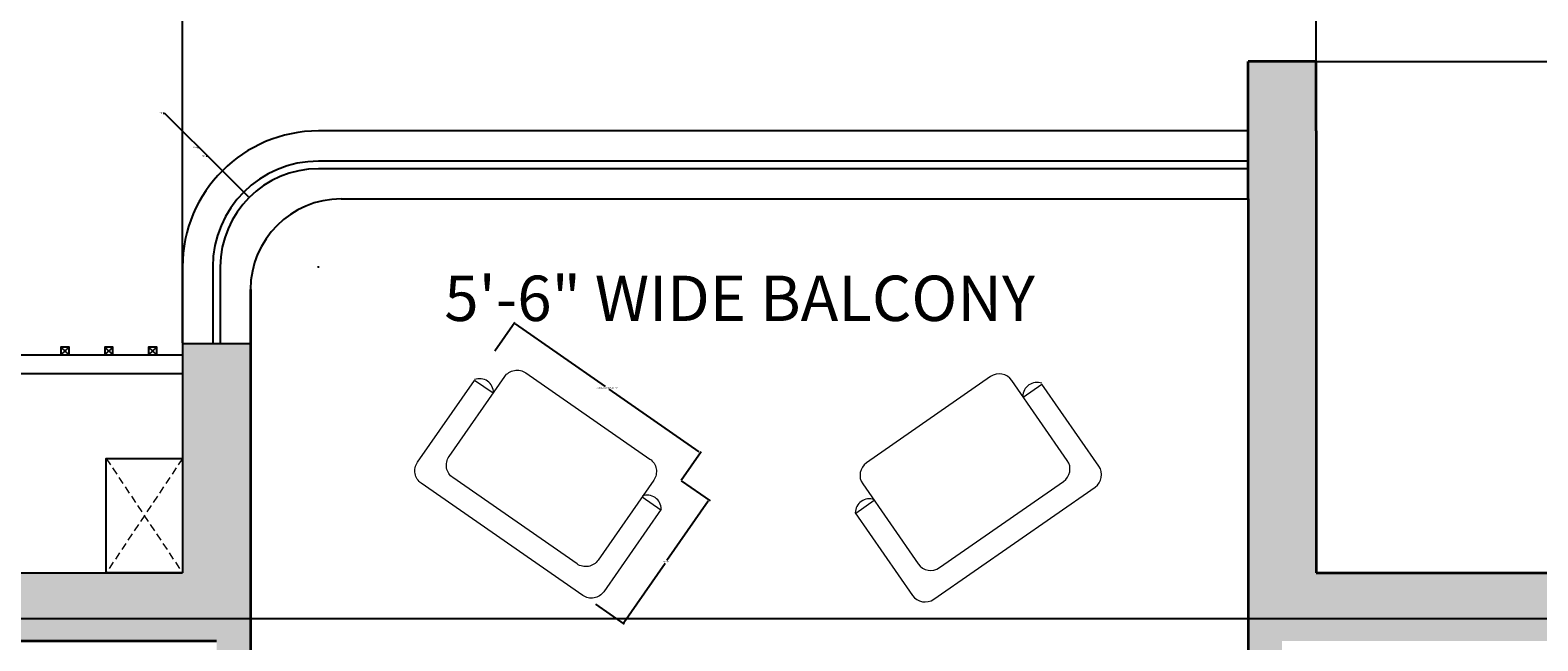
# Model space of a CAD drawing. Units: inches. Extents: x 1693 to 2974, y 2201 to 2965.
# Tile 13 of 24: x 1976 to 2175, y 2698 to 2779. Entities that reach past the tile are written whole.
import ezdxf

# ---------------------------------------------------------------- set-up
doc = ezdxf.new("R2010")
doc.units = ezdxf.units.IN
doc.header["$LTSCALE"] = 2
doc.header["$MEASUREMENT"] = 0
doc.linetypes.add('HIDDEN', pattern=[0.375, 0.25, -0.125])
for name, color, linetype, lineweight in [('A-ANNO-DIMS', 2, 'Continuous', 18), ('A-AREA-IDEN', 7, 'Continuous', 18), ('A-FLOR-RAIL', 7, 'Continuous', 25), ('A-FLOR-SHFT', 7, 'Continuous', 25), ('A-FLOR-SHFT-HIDN', 8, 'HIDDEN', 13), ('A-FURN', 8, 'Continuous', 18), ('A-WALL', 7, 'Continuous', 35)]:
    doc.layers.add(name, color=color, linetype=linetype, lineweight=lineweight)
doc.layers.add('A-WALL-PATT', color=251, linetype='Continuous', lineweight=13, true_color=0x636466)
doc.styles.get("Standard").update_dxf_attribs({"font": 'arial.ttf'})
doc.dimstyles.get("Standard").update_dxf_attribs({"dimtxt": 0.18, "dimasz": 0.18, "dimexe": 0.18, "dimexo": 0.0625, "dimgap": 0.09, "dimtad": 0, "dimtih": 1, "dimtoh": 1, "dimdec": 1, "dimzin": 0, "dimdsep": 46, "dimlunit": 3, "dimtxsty": 'Standard', "dimcen": 0.09, "dimadec": 0, "dimazin": 0, "dimtfac": 1, "dimtdec": 1, "dimtofl": 0, "dimtmove": 0, "dimatfit": 3, "dimfxl": 1, "dimtolj": 1, "dimtzin": 0, "dimarcsym": 0})

# ---------------------------------------------------------------- blocks, each defined once
blk = doc.blocks.new('LOUNGE-CHAIR-A')
at = {"ltscale": 2}
for p, q in [((15.21, 27.01), (15.21, 30.01)), ((15.21, 3), (15.21, 0))]:
    blk.add_line(p, q, dxfattribs=at)
for points in [[(15.31, 0), (2, 0, -0.414214), (0, 2), (0, 28.01, -0.414214), (2, 30.01), (15.21, 30.01)], [(19.9, 5, -0.414214), (17.9, 3), (5, 3, -0.414214), (3, 5), (3, 25.01, -0.414214), (5, 27.01), (17.9, 27.01, -0.414214), (19.9, 25.01), (19.9, 5)]]:
    blk.add_lwpolyline(points, format="xyb", dxfattribs=at)
for centre in [(14.24, 28.53), (14.24, 1.52)]:
    blk.add_arc(centre, 1.86, 305.0084, 54.9916, dxfattribs=at)
blk = doc.blocks.new('SHAFT-GUARD-POST-A')
for p, q in [((1.07, 1.01), (0, 0)), ((0, 1.01), (1.07, 0))]:
    blk.add_line(p, q)
blk.add_lwpolyline([(0, 0), (1.07, 0), (1.07, 1.01), (0, 1.01)], close=True)
blk = doc.blocks.new('*D65')
at = {"layer": 'A-ANNO-DIMS', "color": 0, "lineweight": -2, "ltscale": 2, "transparency": 16777216}
for p, q in [((2037.05, 2736.25), (2039.69, 2740.05)), ((2039.74, 2739.8), (2051.66, 2731.51)), ((2064.12, 2722.86), (2052.19, 2731.14)), ((2061.73, 2719.1), (2064.37, 2722.9))]:
    blk.add_line(p, q, dxfattribs=at)
at = {"layer": 'A-ANNO-DIMS', "color": 0, "ltscale": 2, "transparency": 16777216}
for points in [[(2039.75, 2739.82), (2039.72, 2739.77), (2039.59, 2739.9)], [(2064.13, 2722.88), (2064.1, 2722.83), (2064.26, 2722.75)]]:
    blk.add_solid(points, dxfattribs=at)
at = {"layer": 'Defpoints', "color": 0, "ltscale": 2, "transparency": 16777216}
for p in [(2039.59, 2739.9), (2037.02, 2736.2), (2061.69, 2719.05)]:
    blk.add_point(p, dxfattribs=at)
at = {"layer": 'A-ANNO-DIMS', "color": 0, "ltscale": 2, "transparency": 16777216, "insert": (2051.93, 2731.33), "char_height": 0.18, "attachment_point": 5}
blk.add_mtext('\\A1;LOUNGE CHAIR A 30 TYP.', dxfattribs=at)
blk = doc.blocks.new('*D66')
at = {"layer": 'A-ANNO-DIMS', "color": 0, "lineweight": -2, "ltscale": 2, "transparency": 16777216}
for p, q in [((2061.74, 2719.02), (2065.54, 2716.38)), ((2065.29, 2716.33), (2059.84, 2708.49)), ((2054.14, 2700.29), (2059.59, 2708.13)), ((2050.39, 2702.68), (2054.19, 2700.04))]:
    blk.add_line(p, q, dxfattribs=at)
at = {"layer": 'A-ANNO-DIMS', "color": 0, "ltscale": 2, "transparency": 16777216}
for points in [[(2065.27, 2716.35), (2065.32, 2716.31), (2065.39, 2716.48)], [(2054.12, 2700.31), (2054.17, 2700.27), (2054.04, 2700.14)]]:
    blk.add_solid(points, dxfattribs=at)
at = {"layer": 'Defpoints', "color": 0, "ltscale": 2, "transparency": 16777216}
for p in [(2061.69, 2719.05), (2065.39, 2716.48), (2050.34, 2702.71)]:
    blk.add_point(p, dxfattribs=at)
at = {"layer": 'A-ANNO-DIMS', "color": 0, "ltscale": 2, "transparency": 16777216, "insert": (2059.72, 2708.31), "char_height": 0.18, "attachment_point": 5}
blk.add_mtext('\\A1;20 TYP.', dxfattribs=at)
blk = doc.blocks.new('*D81')
at = {"layer": 'A-ANNO-DIMS', "color": 0, "lineweight": -2, "ltscale": 2, "transparency": 16777216}
for p, q in [((1752.34, 2553.91), (1752.34, 2964.96)), ((1752.52, 2964.78), (2332.94, 2964.78)), ((2914.06, 2964.78), (2333.64, 2964.78)), ((2914.24, 2754.97), (2914.24, 2964.96))]:
    blk.add_line(p, q, dxfattribs=at)
at = {"layer": 'A-ANNO-DIMS', "color": 0, "ltscale": 2, "transparency": 16777216}
for points in [[(1752.52, 2964.81), (1752.52, 2964.75), (1752.34, 2964.78)], [(2914.06, 2964.81), (2914.06, 2964.75), (2914.24, 2964.78)]]:
    blk.add_solid(points, dxfattribs=at)
at = {"layer": 'Defpoints', "color": 0, "ltscale": 2, "transparency": 16777216}
for p in [(2914.24, 2964.78), (2914.24, 2754.9), (1752.34, 2553.84)]:
    blk.add_point(p, dxfattribs=at)
at = {"layer": 'A-ANNO-DIMS', "color": 0, "ltscale": 2, "transparency": 16777216, "insert": (2333.29, 2964.78), "char_height": 0.18, "attachment_point": 5}
blk.add_mtext('\\A1;1162', dxfattribs=at)
blk = doc.blocks.new('*D82')
at = {"layer": 'A-ANNO-DIMS', "color": 0, "lineweight": -2, "ltscale": 2, "transparency": 16777216}
for p, q in [((2615.67, 2906.08), (1693.46, 2906.08)), ((1693.64, 2905.9), (1693.64, 2582.94)), ((1693.64, 2259.62), (1693.64, 2582.58)), ((2096.17, 2259.44), (1693.46, 2259.44))]:
    blk.add_line(p, q, dxfattribs=at)
at = {"layer": 'A-ANNO-DIMS', "color": 0, "ltscale": 2, "transparency": 16777216}
for points in [[(1693.61, 2905.9), (1693.67, 2905.9), (1693.64, 2906.08)], [(1693.61, 2259.62), (1693.67, 2259.62), (1693.64, 2259.44)]]:
    blk.add_solid(points, dxfattribs=at)
at = {"layer": 'Defpoints', "color": 0, "ltscale": 2, "transparency": 16777216}
for p in [(1693.64, 2906.08), (2615.74, 2906.08), (2096.24, 2259.44)]:
    blk.add_point(p, dxfattribs=at)
at = {"layer": 'A-ANNO-DIMS', "color": 0, "ltscale": 2, "transparency": 16777216, "insert": (1693.64, 2582.76), "char_height": 0.18, "attachment_point": 5}
blk.add_mtext('\\A1;646.6', dxfattribs=at)
blk = doc.blocks.new('*D88')
at = {"layer": 'A-ANNO-DIMS', "color": 0, "lineweight": -2, "ltscale": 2, "transparency": 16777216}
for p, q in [((2479.17, 2700.75), (1693.46, 2700.75)), ((1693.64, 2700.57), (1693.64, 2666.44)), ((1693.64, 2631.93), (1693.64, 2666.07)), ((2479.17, 2631.75), (1693.46, 2631.75))]:
    blk.add_line(p, q, dxfattribs=at)
at = {"layer": 'A-ANNO-DIMS', "color": 0, "ltscale": 2, "transparency": 16777216}
for points in [[(1693.61, 2700.57), (1693.67, 2700.57), (1693.64, 2700.75)], [(1693.61, 2631.93), (1693.67, 2631.93), (1693.64, 2631.75)]]:
    blk.add_solid(points, dxfattribs=at)
at = {"layer": 'Defpoints', "color": 0, "ltscale": 2, "transparency": 16777216}
for p in [(1693.64, 2700.75), (2479.24, 2700.75), (2479.24, 2631.75)]:
    blk.add_point(p, dxfattribs=at)
at = {"layer": 'A-ANNO-DIMS', "color": 0, "ltscale": 2, "transparency": 16777216, "insert": (1693.64, 2666.25), "char_height": 0.18, "attachment_point": 5}
blk.add_mtext('\\A1;69', dxfattribs=at)
blk = doc.blocks.new('*D90')
at = {"layer": 'A-ANNO-DIMS', "color": 0, "lineweight": -2, "ltscale": 2, "transparency": 16777216}
for p, q in [((2145.8, 2774.54), (2973.12, 2774.54)), ((2972.94, 2774.36), (2972.94, 2740.87)), ((2972.94, 2707.02), (2972.94, 2740.51)), ((2294.3, 2706.84), (2973.12, 2706.84))]:
    blk.add_line(p, q, dxfattribs=at)
at = {"layer": 'A-ANNO-DIMS', "color": 0, "ltscale": 2, "transparency": 16777216}
for points in [[(2972.91, 2774.36), (2972.97, 2774.36), (2972.94, 2774.54)], [(2972.91, 2707.02), (2972.97, 2707.02), (2972.94, 2706.84)]]:
    blk.add_solid(points, dxfattribs=at)
at = {"layer": 'Defpoints', "color": 0, "ltscale": 2, "transparency": 16777216}
for p in [(2145.74, 2774.54), (2294.24, 2706.84), (2972.94, 2706.84)]:
    blk.add_point(p, dxfattribs=at)
at = {"layer": 'A-ANNO-DIMS', "color": 0, "ltscale": 2, "transparency": 16777216, "insert": (2972.94, 2740.69), "char_height": 0.18, "attachment_point": 5}
blk.add_mtext('\\A1;67.7', dxfattribs=at)
blk = doc.blocks.new('*D103')
at = {"layer": 'A-ANNO-DIMS', "color": 0, "lineweight": -2, "ltscale": 2, "transparency": 16777216}
for p, q in [((1923.74, 2737.28), (1923.74, 2964.96)), ((1923.92, 2964.78), (1959.52, 2964.78)), ((1995.56, 2964.78), (1959.95, 2964.78)), ((1995.74, 2737.28), (1995.74, 2964.96))]:
    blk.add_line(p, q, dxfattribs=at)
at = {"layer": 'A-ANNO-DIMS', "color": 0, "ltscale": 2, "transparency": 16777216}
for points in [[(1923.92, 2964.81), (1923.92, 2964.75), (1923.74, 2964.78)], [(1995.56, 2964.81), (1995.56, 2964.75), (1995.74, 2964.78)]]:
    blk.add_solid(points, dxfattribs=at)
at = {"layer": 'Defpoints', "color": 0, "ltscale": 2, "transparency": 16777216}
for p in [(1995.74, 2964.78), (1923.74, 2737.22), (1995.74, 2737.22)]:
    blk.add_point(p, dxfattribs=at)
at = {"layer": 'A-ANNO-DIMS', "color": 0, "ltscale": 2, "transparency": 16777216, "insert": (1959.74, 2964.78), "char_height": 0.18, "attachment_point": 5}
blk.add_mtext('\\A1;72', dxfattribs=at)
blk = doc.blocks.new('*D104')
at = {"layer": 'A-ANNO-DIMS', "color": 0, "lineweight": -2, "ltscale": 2, "transparency": 16777216}
for p, q in [((1995.74, 2747.41), (1995.74, 2964.96)), ((1995.92, 2964.78), (2070.46, 2964.78)), ((2145.56, 2964.78), (2071.02, 2964.78)), ((2145.74, 2774.6), (2145.74, 2964.96))]:
    blk.add_line(p, q, dxfattribs=at)
at = {"layer": 'A-ANNO-DIMS', "color": 0, "ltscale": 2, "transparency": 16777216}
for points in [[(1995.92, 2964.81), (1995.92, 2964.75), (1995.74, 2964.78)], [(2145.56, 2964.81), (2145.56, 2964.75), (2145.74, 2964.78)]]:
    blk.add_solid(points, dxfattribs=at)
at = {"layer": 'Defpoints', "color": 0, "ltscale": 2, "transparency": 16777216}
for p in [(2145.74, 2964.78), (2145.74, 2774.54), (1995.74, 2747.34)]:
    blk.add_point(p, dxfattribs=at)
at = {"layer": 'A-ANNO-DIMS', "color": 0, "ltscale": 2, "transparency": 16777216, "insert": (2070.74, 2964.78), "char_height": 0.18, "attachment_point": 5}
blk.add_mtext('\\A1;150', dxfattribs=at)
blk = doc.blocks.new('*D109')
at = {"layer": 'A-ANNO-DIMS', "color": 0, "lineweight": -2, "ltscale": 2, "transparency": 16777216}
for p, q in [((1993.19, 2767.71), (1993.37, 2767.71)), ((1993.37, 2767.71), (2000.88, 2760.2)), ((2013.65, 2747.34), (2013.83, 2747.34)), ((2013.74, 2747.25), (2013.74, 2747.43))]:
    blk.add_line(p, q, dxfattribs=at)
at = {"layer": 'A-ANNO-DIMS', "color": 0, "ltscale": 2, "transparency": 16777216}
blk.add_solid([(2000.9, 2760.22), (2000.86, 2760.18), (2001.01, 2760.07)], dxfattribs=at)
at = {"layer": 'Defpoints', "color": 0, "ltscale": 2, "transparency": 16777216}
for p in [(2001.01, 2760.07), (2013.74, 2747.34)]:
    blk.add_point(p, dxfattribs=at)
at = {"layer": 'A-ANNO-DIMS', "color": 0, "ltscale": 2, "transparency": 16777216, "insert": (1992.89, 2767.71), "char_height": 0.18, "attachment_point": 5}
blk.add_mtext('\\A1;R18', dxfattribs=at)
blk = doc.blocks.new('*D110')
at = {"layer": 'A-ANNO-DIMS', "color": 0, "lineweight": -2, "ltscale": 2, "transparency": 16777216}
for p, q in [((1997.72, 2763.18), (1997.9, 2763.18)), ((1997.9, 2763.18), (2003.71, 2757.37)), ((2013.65, 2747.34), (2013.83, 2747.34)), ((2013.74, 2747.25), (2013.74, 2747.43))]:
    blk.add_line(p, q, dxfattribs=at)
at = {"layer": 'A-ANNO-DIMS', "color": 0, "ltscale": 2, "transparency": 16777216}
blk.add_solid([(2003.73, 2757.39), (2003.69, 2757.35), (2003.84, 2757.24)], dxfattribs=at)
at = {"layer": 'Defpoints', "color": 0, "ltscale": 2, "transparency": 16777216}
for p in [(2003.84, 2757.24), (2013.74, 2747.34)]:
    blk.add_point(p, dxfattribs=at)
at = {"layer": 'A-ANNO-DIMS', "color": 0, "ltscale": 2, "transparency": 16777216, "insert": (1997.41, 2763.18), "char_height": 0.18, "attachment_point": 5}
blk.add_mtext('\\A1;R14', dxfattribs=at)
blk = doc.blocks.new('*D111')
at = {"layer": 'A-ANNO-DIMS', "color": 0, "lineweight": -2, "ltscale": 2, "transparency": 16777216}
for p, q in [((1998.85, 2762.05), (1999.03, 2762.05)), ((1999.03, 2762.05), (2004.42, 2756.66)), ((2013.65, 2747.34), (2013.83, 2747.34)), ((2013.74, 2747.25), (2013.74, 2747.43))]:
    blk.add_line(p, q, dxfattribs=at)
at = {"layer": 'A-ANNO-DIMS', "color": 0, "ltscale": 2, "transparency": 16777216}
blk.add_solid([(2004.44, 2756.69), (2004.4, 2756.64), (2004.54, 2756.54)], dxfattribs=at)
at = {"layer": 'Defpoints', "color": 0, "ltscale": 2, "transparency": 16777216}
for p in [(2004.54, 2756.54), (2013.74, 2747.34)]:
    blk.add_point(p, dxfattribs=at)
at = {"layer": 'A-ANNO-DIMS', "color": 0, "ltscale": 2, "transparency": 16777216, "insert": (1998.54, 2762.05), "char_height": 0.18, "attachment_point": 5}
blk.add_mtext('\\A1;R13', dxfattribs=at)

msp = doc.modelspace()

# ---------------------------------------------------------------- hatches: boundary and pattern name
at = {"layer": 'A-WALL-PATT', "ltscale": 2}
h = msp.add_hatch(color=256, dxfattribs=at)
h.dxf.hatch_style = 1
h.paths.add_polyline_path([(1928.2363, 2733.2161), (1930.9384, 2733.2161), (1930.9384, 2737.2161), (1923.7363, 2737.2161), (1923.7363, 2706.8449), (1908.1286, 2706.8449), (1908.1286, 2697.8449), (1923.7363, 2697.8449), (1923.7363, 2692.8449), (1928.2363, 2692.8449), (1928.2363, 2697.8449), (1949.9863, 2697.8449), (1949.9863, 2706.8449), (1928.2363, 2706.8449)])
h.paths.add_polyline_path([(2004.7363, 2737.2161), (1995.7363, 2737.2161), (1995.7363, 2706.8449), (1985.6374, 2706.8449), (1973.9863, 2706.8449), (1973.9863, 2697.8449), (2000.2363, 2697.8449), (2000.2363, 2686.5348), (2000.3613, 2686.5348), (2000.3613, 2667.0432), (2000.2363, 2601.8449), (1928.2363, 2601.8449), (1928.2363, 2662.8449), (1923.7363, 2662.8449), (1923.7363, 2595.3449), (1928.2363, 2595.3449), (1928.2363, 2597.3449), (2004.7363, 2597.3449), (2004.7363, 2681.3449), (2012.7814, 2681.3449), (2028.7363, 2681.3449), (2028.7363, 2690.3449), (2004.7363, 2690.3449)])
h.paths.add_polyline_path([(2190.9863, 2706.8449), (2184.9863, 2706.8449), (2145.7363, 2706.8449), (2145.7363, 2765.3449), (2145.7363, 2774.5394), (2136.7363, 2774.5394), (2136.7363, 2756.3449), (2136.7363, 2690.3449), (2112.7363, 2690.3449), (2112.7363, 2681.3449), (2136.7363, 2681.3449), (2136.7363, 2597.3449), (2141.2363, 2597.3449), (2141.2363, 2697.8449), (2190.9863, 2697.8449)])
h.paths.add_polyline_path([(1860.1286, 2706.8449), (1782.7363, 2706.8449), (1782.7363, 2621.6433), (1791.7363, 2621.6433), (1791.7363, 2697.8449), (1860.1286, 2697.8449)])
h.paths.add_polyline_path([(1791.7363, 2585.6433), (1782.7363, 2585.6433), (1782.7363, 2562.8449), (1782.7363, 2553.8449), (1752.3363, 2553.8449), (1752.3363, 2544.2586), (1756.3363, 2544.2586), (1756.3363, 2549.3449), (1782.7363, 2549.3449), (1782.7363, 2489.2404), (1782.7363, 2477.5455), (1791.7363, 2477.5455), (1791.7363, 2493.5991), (1791.6113, 2493.5991), (1791.6113, 2513.0907), (1791.6824, 2533.7198, -0.94742783), (1791.7363, 2534.7168), (1791.7363, 2549.3449), (1863.7363, 2549.3449), (1863.7363, 2513.3449), (1866.7363, 2513.3449), (1866.7363, 2549.3449), (1924.7363, 2549.3449), (1924.7363, 2447.3449), (1924.7363, 2442.8449), (1933.7363, 2442.8449), (1933.7363, 2447.3449), (1928.2363, 2447.3449), (1928.2363, 2559.3449), (1923.7363, 2559.3449), (1923.7363, 2553.8449), (1791.7363, 2553.8449), (1791.7363, 2562.8449)])
h.paths.add_polyline_path([(1791.7363, 2442.8449), (1866.7363, 2442.8449), (1866.7363, 2447.3449), (1866.7363, 2483.3449), (1863.7363, 2483.3449), (1863.7363, 2447.3449), (1791.7363, 2447.3449), (1791.7363, 2453.5455), (1782.7363, 2453.5455), (1782.7363, 2447.3449), (1756.3363, 2447.3449), (1756.3363, 2455.7126), (1752.3363, 2455.7126), (1752.3363, 2442.8449), (1782.7363, 2442.8449), (1782.7363, 2403.1922), (1791.7363, 2403.1922)])
h.paths.add_polyline_path([(1930.0781, 2298.8449), (1791.7363, 2298.8449), (1791.7363, 2355.1922), (1782.7363, 2355.1922), (1782.7363, 2289.8449), (1930.0781, 2289.8449)])
h.paths.add_polyline_path([(2624.7363, 2883.2547), (2624.7363, 2902.6165), (2624.7363, 2906.0761), (2615.7363, 2906.0761), (2615.7363, 2892.2547), (2615.7363, 2846.2547), (2578.2363, 2846.2547), (2578.2363, 2837.2547), (2620.2363, 2837.2547), (2620.2363, 2743.2547), (2624.7363, 2743.2547), (2624.7363, 2808.2547), (2648.7363, 2808.2547), (2648.7363, 2817.2547), (2624.7363, 2817.2547)])
h.paths.add_polyline_path([(2530.2363, 2846.2547), (2479.2363, 2846.2547), (2479.2363, 2695.8203), (2488.2363, 2695.8203), (2488.2363, 2700.7547), (2567.2363, 2700.7547), (2567.2363, 2705.2547), (2488.2363, 2705.2547), (2488.2363, 2837.2547), (2530.2363, 2837.2547)])
h.paths.add_polyline_path([(2488.2363, 2487.7547), (2630.2363, 2487.7547, -0.00990191), (2630.2363, 2489.0322), (2630.2363, 2492.2547), (2488.2363, 2492.2547), (2488.2363, 2512.4371), (2479.2363, 2512.4371), (2479.2363, 2334.7547), (2608.9702, 2334.7547), (2608.9702, 2343.7547), (2488.2363, 2343.7547)])
h.paths.add_polyline_path([(2751.7544, 2343.7547), (2672.7363, 2343.7547), (2672.7363, 2409.7547), (2674.7363, 2409.7547), (2674.7363, 2413.7547), (2672.7363, 2413.7547), (2672.7363, 2487.7547), (2732.7363, 2487.7547), (2732.7363, 2413.7547), (2704.7363, 2413.7547), (2704.7363, 2409.7547), (2784.7363, 2409.7547), (2784.7363, 2343.7547), (2775.7544, 2343.7547), (2775.7544, 2334.7547), (2902.2363, 2334.7547), (2902.2363, 2520.7999), (2893.2363, 2520.7999), (2893.2363, 2413.7547), (2856.0145, 2413.7547), (2856.0145, 2409.7547), (2893.2363, 2409.7547), (2893.2363, 2343.7547), (2789.2363, 2343.7547), (2789.2363, 2409.7547), (2819.2363, 2409.7547), (2826.0145, 2409.7547), (2826.0145, 2413.7547), (2789.2363, 2413.7547), (2789.2363, 2492.2547), (2784.7363, 2492.2547), (2784.7363, 2413.7547), (2736.7363, 2413.7547), (2736.7363, 2492.2547), (2672.7363, 2492.2547), (2666.2363, 2492.2547), (2666.2363, 2487.7547), (2668.2363, 2487.7547), (2668.2363, 2343.7547), (2656.9702, 2343.7547), (2656.9702, 2334.7547), (2662.9702, 2334.7547), (2751.7544, 2334.7547)])
h.paths.add_polyline_path([(2902.2363, 2613.7547), (2893.2363, 2613.7547), (2893.2363, 2589.7547), (2785.2363, 2589.7547), (2785.2363, 2661.7547), (2790.2363, 2661.7547), (2790.2363, 2665.2547), (2761.2363, 2665.2547), (2761.2363, 2667.2547), (2756.7363, 2667.2547), (2756.7363, 2661.7547), (2781.2363, 2661.7547), (2781.2363, 2585.7547), (2893.2363, 2585.7547), (2893.2363, 2568.7999), (2902.2363, 2568.7999)])
h.paths.add_polyline_path([(2488.2363, 2671.8203), (2479.2363, 2671.8203), (2479.2363, 2645.2547), (2479.2363, 2623.4598), (2488.2363, 2623.4598), (2488.2363, 2636.2547), (2624.7363, 2636.2547), (2624.7363, 2640.7547), (2603.7363, 2640.7547), (2603.7363, 2700.7547), (2624.7363, 2700.7547), (2624.7363, 2707.2547), (2620.2363, 2707.2547), (2620.2363, 2705.2547), (2597.2363, 2705.2547), (2597.2363, 2700.7547), (2599.2363, 2700.7547), (2599.2363, 2640.7547), (2488.2363, 2640.7547)])
h.paths.add_polyline_path([(2761.2363, 2837.2547), (2803.2363, 2837.2547), (2803.2363, 2846.2547), (2797.2363, 2846.2547), (2765.7363, 2846.2547), (2756.7363, 2846.2547), (2756.7363, 2817.2547), (2732.7363, 2817.2547), (2732.7363, 2808.2547), (2756.7363, 2808.2547), (2756.7363, 2703.2547), (2761.2363, 2703.2547)])
h.paths.add_polyline_path([(2739.7489, 2433.1234), (2786.9181, 2433.1234), (2786.9181, 2455.5122), (2739.7489, 2455.5122)], flags=25)

# ---------------------------------------------------------------- linework, layer by layer
at = {"layer": 'A-FLOR-RAIL'}
for p, q in [((2016.7363, 2756.3449), (2136.7363, 2756.3449)), ((1995.7363, 2737.2161), (2004.7363, 2737.2161))]:
    msp.add_line(p, q, dxfattribs=at)
for points in [[(2136.7363, 2765.3449), (2013.7363, 2765.3449, 0.41421356), (1995.7363, 2747.3449), (1995.7363, 2706.8449)], [(2136.7363, 2761.3449), (2013.7363, 2761.3449, 0.41421356), (1999.7363, 2747.3449), (1999.7363, 2737.2161)], [(2136.7363, 2760.3449), (2013.7363, 2760.3449, 0.41421356), (2000.7363, 2747.3449), (2000.7363, 2737.2161)]]:
    msp.add_lwpolyline(points, format="xyb", dxfattribs=at)
msp.add_arc((2016.7363, 2744.3449), 12, 90, 180, dxfattribs=at)
at = {"layer": 'A-FLOR-SHFT'}
for p, q in [((1930.9384, 2735.7161), (1995.7363, 2735.7161)), ((1928.2363, 2733.2161), (1995.7363, 2733.2161)), ((1928.2363, 2706.8449), (1995.7363, 2706.8449))]:
    msp.add_line(p, q, dxfattribs=at)
msp.add_lwpolyline([(1995.7363, 2706.8449), (1985.6374, 2706.8449), (1985.6374, 2721.9811), (1995.7363, 2721.9811)], close=True, dxfattribs=at)
at = {"layer": 'A-FLOR-SHFT-HIDN', "ltscale": 2}
for p, q in [((1985.6374, 2721.9811), (1995.7363, 2706.8449)), ((1995.7363, 2721.9811), (1985.6374, 2706.8449))]:
    msp.add_line(p, q, dxfattribs=at)
at = {"layer": 'A-FURN', "ltscale": 2}
for p, q in [((2106.9887, 2730.1186), (2109.4523, 2731.8306)), ((2087.2759, 2716.4203), (2084.8123, 2714.7083))]:
    msp.add_line(p, q, dxfattribs=at)
for points in [[(2084.7574, 2714.7872), (2092.351, 2703.8596, 0.41421356), (2095.1347, 2703.3585), (2116.4899, 2718.1982, 0.41421356), (2116.991, 2720.9819), (2109.4523, 2731.8306)], [(2086.2451, 2721.4085, 0.41421356), (2085.744, 2718.6248), (2093.1026, 2708.0352, 0.41421356), (2095.8863, 2707.5341), (2112.3144, 2718.9498, 0.41421356), (2112.8155, 2721.7335), (2105.4568, 2732.3231, 0.41421356), (2102.6731, 2732.8242), (2086.2451, 2721.4085)]]:
    msp.add_lwpolyline(points, format="xyb", dxfattribs=at)
for centre in [(2108.7926, 2730.1906), (2086.6162, 2714.7803)]:
    msp.add_arc(centre, 1.8587, 69.803699, 179.786833, dxfattribs=at)
at = {"layer": 'A-WALL'}
for p, q in [((2136.7363, 2756.3449), (2136.7363, 2774.5394)), ((2145.7363, 2774.5394), (2136.7363, 2774.5394)), ((2145.7363, 2765.3449), (2145.7363, 2774.5394)), ((2145.7363, 2765.3449), (2145.7363, 2706.8449)), ((2136.7363, 2756.3449), (2136.7363, 2690.3449)), ((2004.7363, 2744.3449), (2004.7363, 2690.3449)), ((2145.7363, 2706.8449), (2294.2363, 2706.8449)), ((1928.2363, 2697.8449), (2000.2363, 2697.8449))]:
    msp.add_line(p, q, dxfattribs=at)

# ---------------------------------------------------------------- block references
at = {"layer": 'A-FLOR-SHFT'}
for p in [(1979.652, 2735.716), (1985.452, 2735.716), (1991.252, 2735.716)]:
    msp.add_blockref('SHAFT-GUARD-POST-A', p, dxfattribs=at)
at = {"layer": 'A-FURN', "rotation": 55.20473394941792}
msp.add_blockref('LOUNGE-CHAIR-A', (2050.3393, 2702.713), dxfattribs=at)

# ---------------------------------------------------------------- texts
at = {"layer": 'A-AREA-IDEN', "ltscale": 2, "insert": (2030.3755, 2746.1864), "char_height": 6, "attachment_point": 1}
msp.add_mtext_dynamic_manual_height_columns('5\'-6" WIDE BALCONY', width=108.452746, gutter_width=1, heights=[0], dxfattribs=at)

# ---------------------------------------------------------------- dimensions: what is measured, and where the dimension line sits
at = {"layer": 'A-ANNO-DIMS', "ltscale": 2}
for base, p1, p2, picture, middle in [((2914.2363, 2964.7761), (1752.3363, 2553.8449), (2914.2363, 2754.903), '*D81', (2333.2863, 2964.7761)), ((1995.7363, 2964.7761), (1923.7363, 2737.2161), (1995.7363, 2737.2161), '*D103', (1959.7363, 2964.7761)), ((2145.7363, 2964.7761), (1995.7363, 2747.3449), (2145.7363, 2774.5394), '*D104', (2070.7363, 2964.7761))]:
    dim = msp.add_linear_dim(base=base, p1=p1, p2=p2, dimstyle='Standard', override={"dimdec": 0, "dimlfac": 1, "dimrnd": 0, "dimzin": 0, "dimdsep": 46, "dimlunit": 2}, dxfattribs=at)
    dim.commit()
    dim.dimension.update_dxf_attribs({"geometry": picture, "text_midpoint": middle})
for base, p1, p2, override, picture, middle in [((1693.6363, 2906.0761), (2096.2363, 2259.4449), (2615.7363, 2906.0761), {"dimdec": 1, "dimlfac": 1, "dimrnd": 0, "dimzin": 0, "dimdsep": 46, "dimlunit": 2}, '*D82', (1693.6363, 2582.7605)), ((2972.9363, 2706.8449), (2145.7363, 2774.5394), (2294.2363, 2706.8449), {"dimdec": 1, "dimlfac": 1, "dimrnd": 0, "dimzin": 0, "dimdsep": 46, "dimlunit": 2}, '*D90', (2972.9363, 2740.6922)), ((1693.6363, 2700.7547), (2479.2363, 2631.7547), (2479.2363, 2700.7547), {"dimdec": 0, "dimlfac": 1, "dimrnd": 0, "dimzin": 0, "dimdsep": 46, "dimlunit": 2}, '*D88', (1693.6363, 2666.2547))]:
    dim = msp.add_linear_dim(base=base, p1=p1, p2=p2, angle=90, dimstyle='Standard', override=override, dxfattribs=at)
    dim.commit()
    dim.dimension.update_dxf_attribs({"geometry": picture, "text_midpoint": middle})
for mpoint, picture, middle in [((2001.0083, 2760.0727), '*D109', (1992.8862, 2767.7094)), ((2003.8367, 2757.2443), '*D110', (1997.4123, 2763.1839)), ((2004.5438, 2756.5372), '*D111', (1998.5433, 2762.0526))]:
    dim = msp.add_radius_dim(center=(2013.7363, 2747.3449), mpoint=mpoint, dimstyle='Standard', override={"dimdec": 0, "dimlfac": 1, "dimrnd": 0, "dimzin": 0, "dimdsep": 46, "dimlunit": 2}, dxfattribs=at)
    dim.commit()
    dim.dimension.update_dxf_attribs({"geometry": picture, "text_midpoint": middle, "dimtype": 164})
for base, p1, p2, angle, text, picture, middle in [((2039.5878, 2739.9008), (2061.6925, 2719.0514), (2037.0156, 2736.1992), 145.204734, 'LOUNGE CHAIR A <> TYP.', '*D65', (2051.9262, 2731.3268)), ((2065.394, 2716.4792), (2050.3393, 2702.7134), (2061.6925, 2719.0514), 55.204734, '<> TYP.', '*D66', (2059.7174, 2708.3102))]:
    dim = msp.add_linear_dim(base=base, p1=p1, p2=p2, angle=angle, text=text, dimstyle='Standard', override={"dimdec": 0, "dimlfac": 1, "dimrnd": 0, "dimzin": 0, "dimdsep": 46, "dimlunit": 2}, dxfattribs=at)
    dim.commit()
    dim.dimension.update_dxf_attribs({"geometry": picture, "text_midpoint": middle})

doc.saveas('drawing.dxf')
